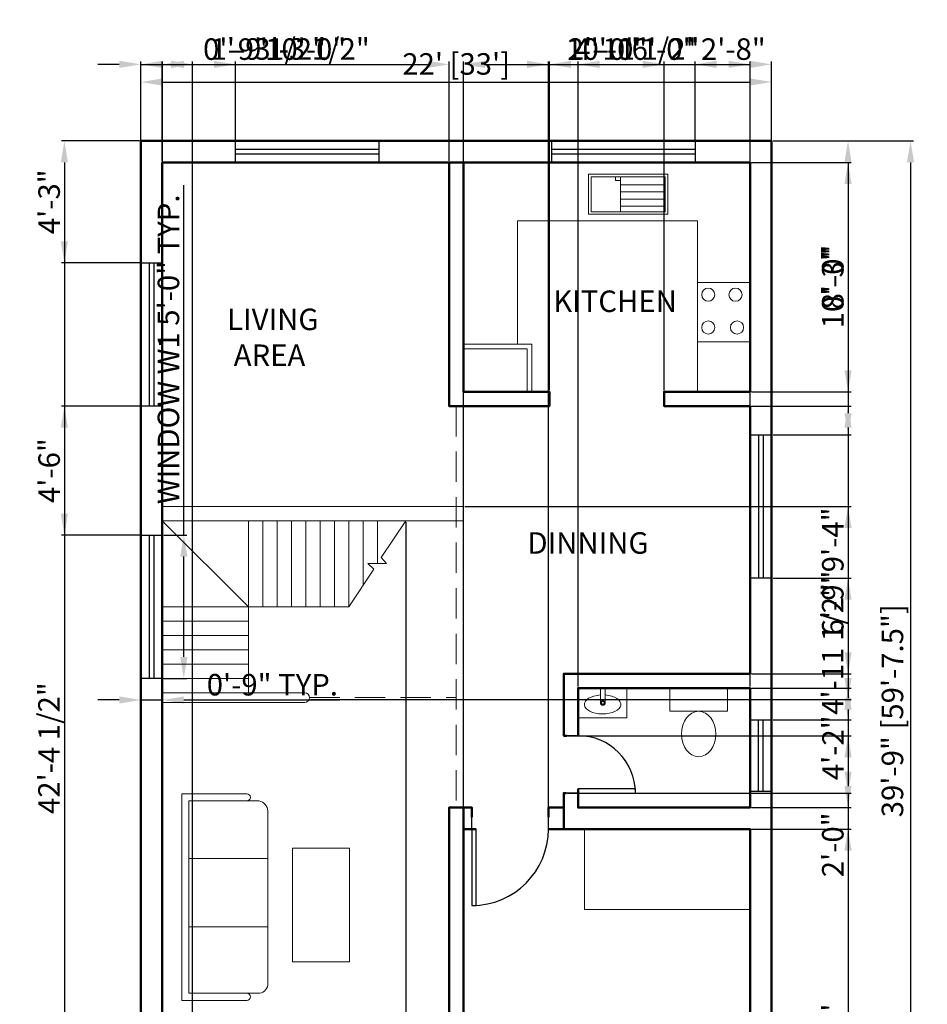
# Model space of a CAD drawing. Units: inches. Extents: x 2429 to 3343, y 1496 to 2530.
# Tile 4 of 7: x 2429 to 2809, y 2118 to 2530. Entities that reach past the tile are written whole.
import ezdxf

# ---------------------------------------------------------------- set-up
doc = ezdxf.new("R2010")
doc.units = ezdxf.units.IN
doc.linetypes.add('DASHED', pattern=[19.05, 12.7, -6.35])
for name, color, linetype, lineweight in [('A-ANNO-DIMS', 2, 'Continuous', 18), ('A-AREA-IDEN', 3, 'Continuous', 18), ('A-DOOR', 3, 'Continuous', 25), ('A-FLOR-FIXT', 8, 'Continuous', 18), ('A-FLOR-OVHD', 8, 'DASHED', 18), ('A-FLOR-STRS', 2, 'Continuous', 18), ('A-FURN', 9, 'Continuous', 18), ('A-GLAZ', 4, 'Continuous', 25), ('A-WALL', 7, 'Continuous', 50)]:
    doc.layers.add(name, color=color, linetype=linetype, lineweight=lineweight)
doc.styles.get("Standard").update_dxf_attribs({"font": 'arial.ttf'})
doc.dimstyles.new('ISO-25', dxfattribs={"dimtxt": 9, "dimasz": 9, "dimexe": 1.25, "dimexo": 0.625, "dimtad": 1, "dimdec": 1, "dimlunit": 3, "dimtxsty": 'Standard', "dimcen": 9, "dimadec": 0, "dimazin": 0, "dimtfac": 1, "dimtdec": 1, "dimtmove": 0, "dimatfit": 3, "dimfxl": 1, "dimarcsym": 0})

# ---------------------------------------------------------------- blocks, each defined once
blk = doc.blocks.new('*U3')
for p, q in [((0, 0), (0, 5)), ((32, 0), (32, 5))]:
    blk.add_line(p, q)
blk.add_lwpolyline([(0, 0), (0, -32), (1.75, -32), (1.75, 0)], close=True)
blk.add_arc((0, 0), 32, 270, 0)
blk = doc.blocks.new('*U4')
for p, q in [((0, 0), (0, 5)), ((24, 0), (24, 5))]:
    blk.add_line(p, q)
blk.add_lwpolyline([(0, 0), (0, -24), (1.75, -24), (1.75, 0)], close=True)
blk.add_arc((0, 0), 24, 270, 0)
blk = doc.blocks.new('*D6')
at = {"layer": 'A-ANNO-DIMS', "color": 0, "lineweight": -2, "transparency": 16777216}
for p, q in [((2479.77, 2480.38), (2479.77, 2505.63)), ((2743.77, 2480.38), (2743.77, 2505.63)), ((2488.77, 2504.38), (2734.77, 2504.38))]:
    blk.add_line(p, q, dxfattribs=at)
at = {"layer": 'A-ANNO-DIMS', "color": 0, "transparency": 16777216}
for points in [[(2488.77, 2505.88), (2488.77, 2502.88), (2479.77, 2504.38)], [(2734.77, 2505.88), (2734.77, 2502.88), (2743.77, 2504.38)]]:
    blk.add_solid(points, dxfattribs=at)
at = {"layer": 'Defpoints', "color": 0, "transparency": 16777216}
for p in [(2743.77, 2504.38), (2479.77, 2479.76), (2743.77, 2479.76)]:
    blk.add_point(p, dxfattribs=at)
at = {"layer": 'A-ANNO-DIMS', "color": 0, "transparency": 16777216, "insert": (2611.77, 2510.77), "char_height": 9, "attachment_point": 5}
blk.add_mtext("22' [33']", dxfattribs=at)
blk = doc.blocks.new('*D7')
at = {"layer": 'A-ANNO-DIMS', "color": 0, "lineweight": -2, "transparency": 16777216}
for p, q in [((2744.82, 2479.76), (2803.17, 2479.76)), ((2801.92, 2470.76), (2801.92, 2011.75)), ((2744.4, 2002.75), (2803.17, 2002.75))]:
    blk.add_line(p, q, dxfattribs=at)
at = {"layer": 'A-ANNO-DIMS', "color": 0, "transparency": 16777216}
for points in [[(2800.42, 2470.76), (2803.42, 2470.76), (2801.92, 2479.76)], [(2800.42, 2011.75), (2803.42, 2011.75), (2801.92, 2002.75)]]:
    blk.add_solid(points, dxfattribs=at)
at = {"layer": 'Defpoints', "color": 0, "transparency": 16777216}
for p in [(2744.19, 2479.76), (2743.77, 2002.75), (2801.92, 2002.75)]:
    blk.add_point(p, dxfattribs=at)
at = {"layer": 'A-ANNO-DIMS', "color": 0, "transparency": 16777216, "insert": (2795.52, 2241.25), "char_height": 9, "attachment_point": 5, "rotation": 90}
blk.add_mtext('39\'-9" [59\'-7.5"]', dxfattribs=at)
blk = doc.blocks.new('WIN-PLAN-1500')
for p, q in [((3.5, 60), (3.5, 0)), ((5.5, 60), (5.5, 0))]:
    blk.add_line(p, q)
blk.add_lwpolyline([(9, 60), (9, 0), (0, 0), (0, 60)], close=True)
blk = doc.blocks.new('WIN-PLAN-750')
for p, q in [((3.5, 0), (3.5, 30)), ((5.5, 0), (5.5, 30))]:
    blk.add_line(p, q)
blk.add_lwpolyline([(9, 30), (9, 0), (0, 0), (0, 30)], close=True)
blk = doc.blocks.new('*D25')
at = {"layer": 'A-ANNO-DIMS', "color": 0, "lineweight": -2, "transparency": 16777216}
for p, q in [((2497.77, 2314.75), (2497.77, 2461.24)), ((2489.4, 2314.75), (2499.02, 2314.75)), ((2497.77, 2263.75), (2497.77, 2305.75)), ((2489.4, 2254.75), (2499.02, 2254.75))]:
    blk.add_line(p, q, dxfattribs=at)
at = {"layer": 'A-ANNO-DIMS', "color": 0, "transparency": 16777216}
for points in [[(2496.27, 2305.75), (2499.27, 2305.75), (2497.77, 2314.75)], [(2496.27, 2263.75), (2499.27, 2263.75), (2497.77, 2254.75)]]:
    blk.add_solid(points, dxfattribs=at)
at = {"layer": 'Defpoints', "color": 0, "transparency": 16777216}
for p in [(2488.77, 2314.75), (2497.77, 2314.75), (2488.77, 2254.75)]:
    blk.add_point(p, dxfattribs=at)
at = {"layer": 'A-ANNO-DIMS', "color": 0, "transparency": 16777216, "insert": (2492.49, 2392.5), "char_height": 9, "attachment_point": 5, "rotation": 90}
blk.add_mtext('WINDOW W1 5\'-0" TYP.', dxfattribs=at)
blk = doc.blocks.new('*D26')
at = {"layer": 'A-ANNO-DIMS', "color": 0, "lineweight": -2, "transparency": 16777216}
for p, q in [((2479.77, 2254.13), (2479.77, 2244.5)), ((2488.77, 2254.13), (2488.77, 2244.5)), ((2470.77, 2245.75), (2461.77, 2245.75)), ((2479.77, 2245.75), (2488.77, 2245.75)), ((2497.77, 2245.75), (2562.88, 2245.75))]:
    blk.add_line(p, q, dxfattribs=at)
at = {"layer": 'A-ANNO-DIMS', "color": 0, "transparency": 16777216}
for points in [[(2470.77, 2247.25), (2470.77, 2244.25), (2479.77, 2245.75)], [(2497.77, 2247.25), (2497.77, 2244.25), (2488.77, 2245.75)]]:
    blk.add_solid(points, dxfattribs=at)
at = {"layer": 'Defpoints', "color": 0, "transparency": 16777216}
for p in [(2479.77, 2254.75), (2488.77, 2254.75), (2488.77, 2245.75)]:
    blk.add_point(p, dxfattribs=at)
at = {"layer": 'A-ANNO-DIMS', "color": 0, "transparency": 16777216, "insert": (2534.83, 2250.97), "char_height": 9, "attachment_point": 5}
blk.add_mtext('0\'-9" TYP.', dxfattribs=at)
blk = doc.blocks.new('*D29')
at = {"layer": 'A-ANNO-DIMS', "color": 0, "lineweight": -2, "transparency": 16777216}
for p, q in [((2479.15, 2479.76), (2446.52, 2479.76)), ((2447.77, 2470.76), (2447.77, 1980.44)), ((2479.15, 1971.44), (2446.52, 1971.44))]:
    blk.add_line(p, q, dxfattribs=at)
at = {"layer": 'A-ANNO-DIMS', "color": 0, "transparency": 16777216}
for points in [[(2446.27, 2470.76), (2449.27, 2470.76), (2447.77, 2479.76)], [(2446.27, 1980.44), (2449.27, 1980.44), (2447.77, 1971.44)]]:
    blk.add_solid(points, dxfattribs=at)
at = {"layer": 'Defpoints', "color": 0, "transparency": 16777216}
for p in [(2479.77, 2479.76), (2447.77, 1971.44), (2479.77, 1971.44)]:
    blk.add_point(p, dxfattribs=at)
at = {"layer": 'A-ANNO-DIMS', "color": 0, "transparency": 16777216, "insert": (2442.49, 2225.6), "char_height": 9, "attachment_point": 5, "rotation": 90}
blk.add_mtext('42\'-4 1/2"', dxfattribs=at)
blk = doc.blocks.new('*D30')
at = {"layer": 'A-ANNO-DIMS', "color": 0, "lineweight": -2, "transparency": 16777216}
for p, q in [((2488.77, 2471.38), (2488.77, 2513.01)), ((2497.77, 2511.76), (2599.77, 2511.76)), ((2608.77, 2471.38), (2608.77, 2513.01))]:
    blk.add_line(p, q, dxfattribs=at)
at = {"layer": 'A-ANNO-DIMS', "color": 0, "transparency": 16777216}
for points in [[(2497.77, 2513.26), (2497.77, 2510.26), (2488.77, 2511.76)], [(2599.77, 2513.26), (2599.77, 2510.26), (2608.77, 2511.76)]]:
    blk.add_solid(points, dxfattribs=at)
at = {"layer": 'Defpoints', "color": 0, "transparency": 16777216}
for p in [(2608.77, 2511.76), (2488.77, 2470.76), (2608.77, 2470.76)]:
    blk.add_point(p, dxfattribs=at)
at = {"layer": 'A-ANNO-DIMS', "color": 0, "transparency": 16777216, "insert": (2548.77, 2516.98), "char_height": 9, "attachment_point": 5}
blk.add_mtext('10\'-0"', dxfattribs=at)
blk = doc.blocks.new('*D31')
at = {"layer": 'A-ANNO-DIMS', "color": 0, "lineweight": -2, "transparency": 16777216}
for p, q in [((2614.77, 2471.38), (2614.77, 2513.01)), ((2623.77, 2511.76), (2725.77, 2511.76)), ((2734.77, 2471.38), (2734.77, 2513.01))]:
    blk.add_line(p, q, dxfattribs=at)
at = {"layer": 'A-ANNO-DIMS', "color": 0, "transparency": 16777216}
for points in [[(2623.77, 2513.26), (2623.77, 2510.26), (2614.77, 2511.76)], [(2725.77, 2513.26), (2725.77, 2510.26), (2734.77, 2511.76)]]:
    blk.add_solid(points, dxfattribs=at)
at = {"layer": 'Defpoints', "color": 0, "transparency": 16777216}
for p in [(2734.77, 2511.76), (2614.77, 2470.76), (2734.77, 2470.76)]:
    blk.add_point(p, dxfattribs=at)
at = {"layer": 'A-ANNO-DIMS', "color": 0, "transparency": 16777216, "insert": (2674.77, 2516.98), "char_height": 9, "attachment_point": 5}
blk.add_mtext('10\'-0"', dxfattribs=at)
blk = doc.blocks.new('*D32')
at = {"layer": 'A-ANNO-DIMS', "color": 0, "lineweight": -2, "transparency": 16777216}
for p, q in [((2735.4, 2470.76), (2777.02, 2470.76)), ((2775.77, 2461.76), (2775.77, 2383.76)), ((2735.4, 2374.76), (2777.02, 2374.76))]:
    blk.add_line(p, q, dxfattribs=at)
at = {"layer": 'A-ANNO-DIMS', "color": 0, "transparency": 16777216}
for points in [[(2774.27, 2461.76), (2777.27, 2461.76), (2775.77, 2470.76)], [(2774.27, 2383.76), (2777.27, 2383.76), (2775.77, 2374.76)]]:
    blk.add_solid(points, dxfattribs=at)
at = {"layer": 'Defpoints', "color": 0, "transparency": 16777216}
for p in [(2734.77, 2470.76), (2734.77, 2374.76), (2775.77, 2374.76)]:
    blk.add_point(p, dxfattribs=at)
at = {"layer": 'A-ANNO-DIMS', "color": 0, "transparency": 16777216, "insert": (2770.55, 2422.76), "char_height": 9, "attachment_point": 5, "rotation": 90}
blk.add_mtext('8\'-0"', dxfattribs=at)
blk = doc.blocks.new('*D33')
at = {"layer": 'A-ANNO-DIMS', "color": 0, "lineweight": -2, "transparency": 16777216}
for p, q in [((2650.77, 2375.38), (2650.77, 2513.01)), ((2659.77, 2511.76), (2689.77, 2511.76)), ((2698.77, 2375.38), (2698.77, 2513.01))]:
    blk.add_line(p, q, dxfattribs=at)
at = {"layer": 'A-ANNO-DIMS', "color": 0, "transparency": 16777216}
for points in [[(2659.77, 2513.26), (2659.77, 2510.26), (2650.77, 2511.76)], [(2689.77, 2513.26), (2689.77, 2510.26), (2698.77, 2511.76)]]:
    blk.add_solid(points, dxfattribs=at)
at = {"layer": 'Defpoints', "color": 0, "transparency": 16777216}
for p in [(2698.77, 2511.76), (2650.77, 2374.76), (2698.77, 2374.76)]:
    blk.add_point(p, dxfattribs=at)
at = {"layer": 'A-ANNO-DIMS', "color": 0, "transparency": 16777216, "insert": (2674.77, 2516.98), "char_height": 9, "attachment_point": 5}
blk.add_mtext('4\'-0"', dxfattribs=at)
blk = doc.blocks.new('*D34')
at = {"layer": 'A-ANNO-DIMS', "color": 0, "lineweight": -2, "transparency": 16777216}
for p, q in [((2590.68, 2320.13), (2590.68, 1870.45)), ((2488.77, 2248.13), (2488.77, 1870.45)), ((2497.77, 1871.7), (2581.68, 1871.7))]:
    blk.add_line(p, q, dxfattribs=at)
at = {"layer": 'A-ANNO-DIMS', "color": 0, "transparency": 16777216}
for points in [[(2497.77, 1873.2), (2497.77, 1870.2), (2488.77, 1871.7)], [(2581.68, 1873.2), (2581.68, 1870.2), (2590.68, 1871.7)]]:
    blk.add_solid(points, dxfattribs=at)
at = {"layer": 'Defpoints', "color": 0, "transparency": 16777216}
for p in [(2590.68, 2320.75), (2488.77, 2248.75), (2590.68, 1871.7)]:
    blk.add_point(p, dxfattribs=at)
at = {"layer": 'A-ANNO-DIMS', "color": 0, "transparency": 16777216, "insert": (2539.73, 1876.92), "char_height": 9, "attachment_point": 5}
blk.add_mtext('8\'-6"', dxfattribs=at)
blk = doc.blocks.new('*D35')
at = {"layer": 'A-ANNO-DIMS', "color": 0, "lineweight": -2, "transparency": 16777216}
for p, q in [((2615.4, 2326.75), (2777.02, 2326.75)), ((2775.77, 2317.75), (2775.77, 2254.97)), ((2550.83, 2245.97), (2777.02, 2245.97))]:
    blk.add_line(p, q, dxfattribs=at)
at = {"layer": 'A-ANNO-DIMS', "color": 0, "transparency": 16777216}
for points in [[(2774.27, 2317.75), (2777.27, 2317.75), (2775.77, 2326.75)], [(2774.27, 2254.97), (2777.27, 2254.97), (2775.77, 2245.97)]]:
    blk.add_solid(points, dxfattribs=at)
at = {"layer": 'Defpoints', "color": 0, "transparency": 16777216}
for p in [(2614.77, 2326.75), (2550.2, 2245.97), (2775.77, 2245.97)]:
    blk.add_point(p, dxfattribs=at)
at = {"layer": 'A-ANNO-DIMS', "color": 0, "transparency": 16777216, "insert": (2770.55, 2286.36), "char_height": 9, "attachment_point": 5, "rotation": 90}
blk.add_mtext('6\'-9"', dxfattribs=at)
blk = doc.blocks.new('*D36')
at = {"layer": 'A-ANNO-DIMS', "color": 0, "lineweight": -2, "transparency": 16777216}
for p, q in [((2662.77, 2251.38), (2662.77, 2513.01)), ((2671.77, 2511.76), (2725.77, 2511.76)), ((2734.77, 2251.38), (2734.77, 2513.01))]:
    blk.add_line(p, q, dxfattribs=at)
at = {"layer": 'A-ANNO-DIMS', "color": 0, "transparency": 16777216}
for points in [[(2671.77, 2513.26), (2671.77, 2510.26), (2662.77, 2511.76)], [(2725.77, 2513.26), (2725.77, 2510.26), (2734.77, 2511.76)]]:
    blk.add_solid(points, dxfattribs=at)
at = {"layer": 'Defpoints', "color": 0, "transparency": 16777216}
for p in [(2734.77, 2511.76), (2662.77, 2250.76), (2734.77, 2250.76)]:
    blk.add_point(p, dxfattribs=at)
at = {"layer": 'A-ANNO-DIMS', "color": 0, "transparency": 16777216, "insert": (2698.77, 2516.98), "char_height": 9, "attachment_point": 5}
blk.add_mtext('6\'-0"', dxfattribs=at)
blk = doc.blocks.new('*D37')
at = {"layer": 'A-ANNO-DIMS', "color": 0, "lineweight": -2, "transparency": 16777216}
for p, q in [((2735.4, 2250.76), (2777.02, 2250.76)), ((2775.77, 2241.76), (2775.77, 2209.75)), ((2735.4, 2200.75), (2777.02, 2200.75))]:
    blk.add_line(p, q, dxfattribs=at)
at = {"layer": 'A-ANNO-DIMS', "color": 0, "transparency": 16777216}
for points in [[(2774.27, 2241.76), (2777.27, 2241.76), (2775.77, 2250.76)], [(2774.27, 2209.75), (2777.27, 2209.75), (2775.77, 2200.75)]]:
    blk.add_solid(points, dxfattribs=at)
at = {"layer": 'Defpoints', "color": 0, "transparency": 16777216}
for p in [(2734.77, 2250.76), (2734.77, 2200.75), (2775.77, 2200.75)]:
    blk.add_point(p, dxfattribs=at)
at = {"layer": 'A-ANNO-DIMS', "color": 0, "transparency": 16777216, "insert": (2770.63, 2225.75), "char_height": 9, "attachment_point": 5, "rotation": 90}
blk.add_mtext('4\'-2"', dxfattribs=at)
blk = doc.blocks.new('*D39')
at = {"layer": 'A-ANNO-DIMS', "color": 0, "lineweight": -2, "transparency": 16777216}
for p, q in [((2735.4, 2191.75), (2777.02, 2191.75)), ((2775.77, 2182.75), (2775.77, 2020.75)), ((2735.4, 2011.75), (2777.02, 2011.75))]:
    blk.add_line(p, q, dxfattribs=at)
at = {"layer": 'A-ANNO-DIMS', "color": 0, "transparency": 16777216}
for points in [[(2774.27, 2182.75), (2777.27, 2182.75), (2775.77, 2191.75)], [(2774.27, 2020.75), (2777.27, 2020.75), (2775.77, 2011.75)]]:
    blk.add_solid(points, dxfattribs=at)
at = {"layer": 'Defpoints', "color": 0, "transparency": 16777216}
for p in [(2734.77, 2191.75), (2734.77, 2011.75), (2775.77, 2011.75)]:
    blk.add_point(p, dxfattribs=at)
at = {"layer": 'A-ANNO-DIMS', "color": 0, "transparency": 16777216, "insert": (2770.55, 2101.75), "char_height": 9, "attachment_point": 5, "rotation": 90}
blk.add_mtext('15\'-0"', dxfattribs=at)
blk = doc.blocks.new('*D40')
at = {"layer": 'A-ANNO-DIMS', "color": 0, "lineweight": -2, "transparency": 16777216}
for p, q in [((2735.4, 2368.76), (2777.02, 2368.76)), ((2775.77, 2359.76), (2775.77, 2265.76)), ((2735.4, 2256.76), (2777.02, 2256.76))]:
    blk.add_line(p, q, dxfattribs=at)
at = {"layer": 'A-ANNO-DIMS', "color": 0, "transparency": 16777216}
for points in [[(2774.27, 2359.76), (2777.27, 2359.76), (2775.77, 2368.76)], [(2774.27, 2265.76), (2777.27, 2265.76), (2775.77, 2256.76)]]:
    blk.add_solid(points, dxfattribs=at)
at = {"layer": 'Defpoints', "color": 0, "transparency": 16777216}
for p in [(2734.77, 2368.76), (2734.77, 2256.76), (2775.77, 2256.76)]:
    blk.add_point(p, dxfattribs=at)
at = {"layer": 'A-ANNO-DIMS', "color": 0, "transparency": 16777216, "insert": (2770.55, 2312.76), "char_height": 9, "attachment_point": 5, "rotation": 90}
blk.add_mtext('9\'-4"', dxfattribs=at)
blk = doc.blocks.new('*D43')
at = {"layer": 'A-ANNO-DIMS', "color": 0, "lineweight": -2, "transparency": 16777216}
for p, q in [((2470.77, 2511.76), (2461.77, 2511.76)), ((2479.77, 1972.06), (2479.77, 2513.01)), ((2479.77, 2511.76), (2488.8, 2511.76)), ((2488.8, 1972.06), (2488.8, 2513.01)), ((2497.8, 2511.76), (2531.97, 2511.76))]:
    blk.add_line(p, q, dxfattribs=at)
at = {"layer": 'A-ANNO-DIMS', "color": 0, "transparency": 16777216}
for points in [[(2470.77, 2513.26), (2470.77, 2510.26), (2479.77, 2511.76)], [(2497.8, 2513.26), (2497.8, 2510.26), (2488.8, 2511.76)]]:
    blk.add_solid(points, dxfattribs=at)
at = {"layer": 'Defpoints', "color": 0, "transparency": 16777216}
for p in [(2488.8, 2511.76), (2479.77, 1971.44), (2488.8, 1971.44)]:
    blk.add_point(p, dxfattribs=at)
at = {"layer": 'A-ANNO-DIMS', "color": 0, "transparency": 16777216, "insert": (2519.38, 2516.98), "char_height": 9, "attachment_point": 5}
blk.add_mtext('0\'-9"', dxfattribs=at)
blk = doc.blocks.new('*D46')
at = {"layer": 'A-ANNO-DIMS', "color": 0, "lineweight": -2, "transparency": 16777216}
for p, q in [((2658.4, 2230.8), (2777.02, 2230.8)), ((2775.77, 2221.8), (2775.77, 2215.8)), ((2658.4, 2206.8), (2777.02, 2206.8)), ((2775.77, 2206.8), (2775.77, 2172.47))]:
    blk.add_line(p, q, dxfattribs=at)
at = {"layer": 'A-ANNO-DIMS', "color": 0, "transparency": 16777216}
for points in [[(2774.27, 2221.8), (2777.27, 2221.8), (2775.77, 2230.8)], [(2774.27, 2215.8), (2777.27, 2215.8), (2775.77, 2206.8)]]:
    blk.add_solid(points, dxfattribs=at)
at = {"layer": 'Defpoints', "color": 0, "transparency": 16777216}
for p in [(2657.77, 2230.8), (2657.77, 2206.8), (2775.77, 2206.8)]:
    blk.add_point(p, dxfattribs=at)
at = {"layer": 'A-ANNO-DIMS', "color": 0, "transparency": 16777216, "insert": (2770.55, 2185.14), "char_height": 9, "attachment_point": 5, "rotation": 90}
blk.add_mtext('2\'-0"', dxfattribs=at)
blk = doc.blocks.new('*D47')
at = {"layer": 'A-ANNO-DIMS', "color": 0, "lineweight": -2, "transparency": 16777216}
for p, q in [((2614.77, 2192.38), (2614.77, 2513.01)), ((2623.77, 2511.76), (2641.37, 2511.76)), ((2650.37, 2192.38), (2650.37, 2513.01)), ((2650.37, 2511.76), (2712.66, 2511.76))]:
    blk.add_line(p, q, dxfattribs=at)
at = {"layer": 'A-ANNO-DIMS', "color": 0, "transparency": 16777216}
for points in [[(2623.77, 2513.26), (2623.77, 2510.26), (2614.77, 2511.76)], [(2641.37, 2513.26), (2641.37, 2510.26), (2650.37, 2511.76)]]:
    blk.add_solid(points, dxfattribs=at)
at = {"layer": 'Defpoints', "color": 0, "transparency": 16777216}
for p in [(2650.37, 2511.76), (2614.77, 2191.75), (2650.37, 2191.75)]:
    blk.add_point(p, dxfattribs=at)
at = {"layer": 'A-ANNO-DIMS', "color": 0, "transparency": 16777216, "insert": (2686.01, 2517.03), "char_height": 9, "attachment_point": 5}
blk.add_mtext('2\'-11 1/2"', dxfattribs=at)
blk = doc.blocks.new('*D48')
at = {"layer": 'A-ANNO-DIMS', "color": 0, "lineweight": -2, "transparency": 16777216}
for p, q in [((2479.77, 2480.38), (2479.77, 2513.01)), ((2488.77, 2511.76), (2510.36, 2511.76)), ((2519.36, 2480.38), (2519.36, 2513.01)), ((2519.36, 2511.76), (2574.5, 2511.76))]:
    blk.add_line(p, q, dxfattribs=at)
at = {"layer": 'A-ANNO-DIMS', "color": 0, "transparency": 16777216}
for points in [[(2488.77, 2513.26), (2488.77, 2510.26), (2479.77, 2511.76)], [(2510.36, 2513.26), (2510.36, 2510.26), (2519.36, 2511.76)]]:
    blk.add_solid(points, dxfattribs=at)
at = {"layer": 'Defpoints', "color": 0, "transparency": 16777216}
for p in [(2519.36, 2511.76), (2479.77, 2479.76), (2519.36, 2479.76)]:
    blk.add_point(p, dxfattribs=at)
at = {"layer": 'A-ANNO-DIMS', "color": 0, "transparency": 16777216, "insert": (2551.43, 2517.04), "char_height": 9, "attachment_point": 5}
blk.add_mtext('3\'-3 1/2"', dxfattribs=at)
blk = doc.blocks.new('*D49')
at = {"layer": 'A-ANNO-DIMS', "color": 0, "lineweight": -2, "transparency": 16777216}
for p, q in [((2711.73, 2480.38), (2711.73, 2513.01)), ((2720.73, 2511.76), (2734.77, 2511.76)), ((2743.77, 2480.38), (2743.77, 2513.01))]:
    blk.add_line(p, q, dxfattribs=at)
at = {"layer": 'A-ANNO-DIMS', "color": 0, "transparency": 16777216}
for points in [[(2720.73, 2513.26), (2720.73, 2510.26), (2711.73, 2511.76)], [(2734.77, 2513.26), (2734.77, 2510.26), (2743.77, 2511.76)]]:
    blk.add_solid(points, dxfattribs=at)
at = {"layer": 'Defpoints', "color": 0, "transparency": 16777216}
for p in [(2743.77, 2511.76), (2711.73, 2479.76), (2743.77, 2479.76)]:
    blk.add_point(p, dxfattribs=at)
at = {"layer": 'A-ANNO-DIMS', "color": 0, "transparency": 16777216, "insert": (2727.75, 2516.98), "char_height": 9, "attachment_point": 5}
blk.add_mtext('2\'-8"', dxfattribs=at)
blk = doc.blocks.new('*D50')
at = {"layer": 'A-ANNO-DIMS', "color": 0, "lineweight": -2, "transparency": 16777216}
for p, q in [((2479.15, 2479.76), (2446.52, 2479.76)), ((2447.77, 2470.76), (2447.77, 2437.75)), ((2479.15, 2428.75), (2446.52, 2428.75))]:
    blk.add_line(p, q, dxfattribs=at)
at = {"layer": 'A-ANNO-DIMS', "color": 0, "transparency": 16777216}
for points in [[(2446.27, 2470.76), (2449.27, 2470.76), (2447.77, 2479.76)], [(2446.27, 2437.75), (2449.27, 2437.75), (2447.77, 2428.75)]]:
    blk.add_solid(points, dxfattribs=at)
at = {"layer": 'Defpoints', "color": 0, "transparency": 16777216}
for p in [(2479.77, 2479.76), (2447.77, 2428.75), (2479.77, 2428.75)]:
    blk.add_point(p, dxfattribs=at)
at = {"layer": 'A-ANNO-DIMS', "color": 0, "transparency": 16777216, "insert": (2442.55, 2454.25), "char_height": 9, "attachment_point": 5, "rotation": 90}
blk.add_mtext('4\'-3"', dxfattribs=at)
blk = doc.blocks.new('*D51')
at = {"layer": 'A-ANNO-DIMS', "color": 0, "lineweight": -2, "transparency": 16777216}
for p, q in [((2479.15, 2368.75), (2446.52, 2368.75)), ((2447.77, 2359.75), (2447.77, 2323.75)), ((2479.15, 2314.75), (2446.52, 2314.75))]:
    blk.add_line(p, q, dxfattribs=at)
at = {"layer": 'A-ANNO-DIMS', "color": 0, "transparency": 16777216}
for points in [[(2446.27, 2359.75), (2449.27, 2359.75), (2447.77, 2368.75)], [(2446.27, 2323.75), (2449.27, 2323.75), (2447.77, 2314.75)]]:
    blk.add_solid(points, dxfattribs=at)
at = {"layer": 'Defpoints', "color": 0, "transparency": 16777216}
for p in [(2479.77, 2368.75), (2447.77, 2314.75), (2479.77, 2314.75)]:
    blk.add_point(p, dxfattribs=at)
at = {"layer": 'A-ANNO-DIMS', "color": 0, "transparency": 16777216, "insert": (2442.55, 2341.75), "char_height": 9, "attachment_point": 5, "rotation": 90}
blk.add_mtext('4\'-6"', dxfattribs=at)
blk = doc.blocks.new('*D52')
at = {"layer": 'A-ANNO-DIMS', "color": 0, "lineweight": -2, "transparency": 16777216}
for p, q in [((2744.4, 2479.76), (2777.02, 2479.76)), ((2775.77, 2470.76), (2775.77, 2365.75)), ((2744.4, 2356.75), (2777.02, 2356.75))]:
    blk.add_line(p, q, dxfattribs=at)
at = {"layer": 'A-ANNO-DIMS', "color": 0, "transparency": 16777216}
for points in [[(2774.27, 2470.76), (2777.27, 2470.76), (2775.77, 2479.76)], [(2774.27, 2365.75), (2777.27, 2365.75), (2775.77, 2356.75)]]:
    blk.add_solid(points, dxfattribs=at)
at = {"layer": 'Defpoints', "color": 0, "transparency": 16777216}
for p in [(2743.77, 2479.76), (2743.77, 2356.75), (2775.77, 2356.75)]:
    blk.add_point(p, dxfattribs=at)
at = {"layer": 'A-ANNO-DIMS', "color": 0, "transparency": 16777216, "insert": (2770.55, 2418.25), "char_height": 9, "attachment_point": 5, "rotation": 90}
blk.add_mtext('10\'-3"', dxfattribs=at)
blk = doc.blocks.new('*D53')
at = {"layer": 'A-ANNO-DIMS', "color": 0, "lineweight": -2, "transparency": 16777216}
for p, q in [((2744.4, 2296.75), (2777.02, 2296.75)), ((2775.77, 2287.75), (2775.77, 2246.46)), ((2744.4, 2237.46), (2777.02, 2237.46))]:
    blk.add_line(p, q, dxfattribs=at)
at = {"layer": 'A-ANNO-DIMS', "color": 0, "transparency": 16777216}
for points in [[(2774.27, 2287.75), (2777.27, 2287.75), (2775.77, 2296.75)], [(2774.27, 2246.46), (2777.27, 2246.46), (2775.77, 2237.46)]]:
    blk.add_solid(points, dxfattribs=at)
at = {"layer": 'Defpoints', "color": 0, "transparency": 16777216}
for p in [(2743.77, 2296.75), (2743.77, 2237.46), (2775.77, 2237.46)]:
    blk.add_point(p, dxfattribs=at)
at = {"layer": 'A-ANNO-DIMS', "color": 0, "transparency": 16777216, "insert": (2770.49, 2267.11), "char_height": 9, "attachment_point": 5, "rotation": 90}
blk.add_mtext('4\'-11 1/2"', dxfattribs=at)
blk = doc.blocks.new('*D54')
at = {"layer": 'A-ANNO-DIMS', "color": 0, "lineweight": -2, "transparency": 16777216}
for p, q in [((2479.77, 2072.38), (2479.77, 2513.01)), ((2488.77, 2511.76), (2492.46, 2511.76)), ((2501.46, 2072.38), (2501.46, 2513.01)), ((2501.46, 2511.76), (2555.76, 2511.76))]:
    blk.add_line(p, q, dxfattribs=at)
at = {"layer": 'A-ANNO-DIMS', "color": 0, "transparency": 16777216}
for points in [[(2488.77, 2513.26), (2488.77, 2510.26), (2479.77, 2511.76)], [(2492.46, 2513.26), (2492.46, 2510.26), (2501.46, 2511.76)]]:
    blk.add_solid(points, dxfattribs=at)
at = {"layer": 'Defpoints', "color": 0, "transparency": 16777216}
for p in [(2501.46, 2511.76), (2479.77, 2071.75), (2501.46, 2071.75)]:
    blk.add_point(p, dxfattribs=at)
at = {"layer": 'A-ANNO-DIMS', "color": 0, "transparency": 16777216, "insert": (2533.11, 2517.03), "char_height": 9, "attachment_point": 5}
blk.add_mtext('1\'-9 1/2"', dxfattribs=at)

msp = doc.modelspace()

# ---------------------------------------------------------------- hatches: boundary and pattern name
at = {"layer": 'A-FLOR-FIXT'}
h = msp.add_hatch(color=256, dxfattribs=at)
h.dxf.hatch_style = 1
h.paths.add_polyline_path([(2672.14515, 2244.52848, 1), (2674.14515, 2244.52848, 1)])
h.paths.add_polyline_path([(2673.70762, 2244.52848, -1), (2672.58269, 2244.52848, -1)], flags=16)

# ---------------------------------------------------------------- linework, layer by layer
for p, q in [((2680.59018, 2464.75512), (2680.59018, 2450.02691)), ((2680.59018, 2461.38243), (2699.28813, 2461.38243)), ((2680.59018, 2458.38243), (2699.28813, 2458.38243)), ((2680.59018, 2455.38243), (2699.28813, 2455.38243)), ((2680.59018, 2452.38243), (2699.28813, 2452.38243)), ((2712.77109, 2420.52216), (2734.77257, 2420.52216)), ((2712.77109, 2395.6064), (2734.77257, 2395.6064))]:
    msp.add_line(p, q, dxfattribs=at)
for points in [[(2667.19363, 2465.75512), (2700.28813, 2465.75512), (2700.28813, 2449.02691), (2667.19363, 2449.02691)], [(2668.19363, 2464.75512), (2699.28813, 2464.75512), (2699.28813, 2450.02691), (2668.19363, 2450.02691)]]:
    msp.add_lwpolyline(points, close=True, dxfattribs=at)
for points in [[(2678.4916, 2464.75512), (2678.4916, 2463.12164), (2680.59018, 2463.12164)], [(2637.41644, 2394.64579), (2637.41644, 2446.29538), (2712.77109, 2446.29538), (2712.77109, 2374.75602)], [(2662.77257, 2238.21467), (2683.19871, 2238.21467), (2683.19871, 2250.75602)], [(2701.18915, 2250.75602), (2701.18915, 2241.03426), (2725.29415, 2241.03426), (2725.29415, 2250.75602)]]:
    msp.add_lwpolyline(points, dxfattribs=at)
msp.add_lwpolyline([(2672.14515, 2250.75602), (2672.14515, 2244.52848, 1), (2674.14515, 2244.52848), (2674.14515, 2250.75602)], format="xyb", dxfattribs=at)
for centre, radius in [((2717.26639, 2415.37019), 2.74723), ((2728.64581, 2415.37019), 2.74723), ((2717.26639, 2401.63403), 2.74723), ((2729.30948, 2401.63403), 2.74723), ((2673.14515, 2244.52848), 1), ((2673.14515, 2244.52848), 0.56247)]:
    msp.add_circle(centre, radius, dxfattribs=at)
msp.add_ellipse((2673.03582, 2243.89542), major_axis=(7.63165, 0), ratio=0.522688861, start_param=1.687769865, end_param=7.708105138, dxfattribs=at)
msp.add_ellipse((2713.24165, 2231.5072), major_axis=(0, -9.52707), ratio=0.757824975, dxfattribs=at)
at = {"layer": 'A-FLOR-OVHD'}
for p, q in [((2611.77257, 2368.75602), (2611.77257, 2200.7507)), ((2550.35753, 2246.7507), (2611.77257, 2246.7507))]:
    msp.add_line(p, q, dxfattribs=at)
at = {"layer": 'A-FLOR-STRS'}
for p, q in [((2524.77257, 2248.7507), (2524.77257, 2320.7507)), ((2530.77257, 2284.7507), (2530.77257, 2320.7507)), ((2536.77257, 2284.7507), (2536.77257, 2320.7507)), ((2542.77257, 2284.7507), (2542.77257, 2320.7507)), ((2548.77257, 2284.7507), (2548.77257, 2320.7507)), ((2554.77257, 2284.7507), (2554.77257, 2320.7507)), ((2560.77257, 2284.7507), (2560.77257, 2320.7507)), ((2572.77257, 2293.78539), (2572.77257, 2320.7507)), ((2566.77257, 2284.7507), (2488.77257, 2284.7507)), ((2488.77257, 2278.7507), (2524.77257, 2278.7507)), ((2488.77257, 2272.7507), (2524.77257, 2272.7507)), ((2488.77257, 2266.7507), (2524.77257, 2266.7507)), ((2488.77257, 2260.7507), (2524.77257, 2260.7507)), ((2488.77257, 2254.7507), (2524.77257, 2254.7507))]:
    msp.add_line(p, q, dxfattribs=at)
for points in [[(2488.77257, 2326.7507), (2608.77257, 2326.7507), (2614.77257, 2326.7507), (2614.77257, 2320.7507), (2488.77257, 2320.7507), (2524.77257, 2284.7507)], [(2578.77257, 2302.82009), (2574.83944, 2302.82009), (2577.24521, 2300.52021), (2566.77257, 2284.7507), (2566.77257, 2320.7507)], [(2578.77257, 2320.7507), (2578.77257, 2302.82009), (2582.63541, 2302.82009), (2580.43357, 2305.32118), (2590.68041, 2320.7507)]]:
    msp.add_lwpolyline(points, dxfattribs=at)
msp.add_lwpolyline([(2488.77257, 2244.7507), (2548.35753, 2244.7507, 1), (2548.35753, 2248.7507), (2488.77257, 2248.7507)], format="xyb", dxfattribs=at)
at = {"layer": 'A-FURN'}
for p, q in [((2499.92065, 2179.38597), (2532.90986, 2179.38597)), ((2499.92065, 2150.7572), (2532.90986, 2150.7572))]:
    msp.add_line(p, q, dxfattribs=at)
for points in [[(2614.77257, 2394.64579), (2643.4489, 2394.64579), (2643.4489, 2374.75602)], [(2614.77257, 2392.64579), (2641.4489, 2392.64579), (2641.4489, 2374.75602)], [(2665.49179, 2191.7507), (2665.49179, 2158.06801), (2734.77257, 2158.06801)]]:
    msp.add_lwpolyline(points, dxfattribs=at)
for points in [[(2524.1217, 2123.03037), (2499.92065, 2123.03037), (2499.92065, 2203.50803), (2524.1217, 2203.50803, 1), (2524.1217, 2206.50803), (2496.92065, 2206.50803), (2496.92065, 2120.03037), (2524.1217, 2120.03037, 1), (2524.1217, 2123.03037), (2529.24812, 2123.03037)], [(2528.76628, 2123.03037, 0.3909175), (2532.90986, 2126.40966), (2532.90986, 2199.29265, 0.341849533), (2529.27871, 2203.50803), (2520.63409, 2203.50803)]]:
    msp.add_lwpolyline(points, format="xyb", dxfattribs=at)
msp.add_lwpolyline([(2543.28451, 2183.72972), (2567.11852, 2183.72972), (2567.11852, 2136.10076), (2543.28451, 2136.10076)], close=True, dxfattribs=at)
at = {"layer": 'A-WALL'}
for points in [[(2603.44497, 2075.7507), (2603.44497, 2071.7507), (2608.77257, 2071.7507), (2608.77257, 2002.7507), (2743.77257, 2002.7507), (2743.77257, 2326.7507), (2743.77257, 2479.75602), (2479.77257, 2479.75602), (2479.77257, 2326.7507), (2479.77257, 2320.7507), (2479.77257, 2200.7507), (2479.77257, 2071.7507), (2567.44497, 2071.7507), (2567.44497, 2073.04361), (2567.44497, 2075.7507)], [(2658.07657, 2230.80141), (2656.77257, 2230.80141), (2656.77257, 2256.75602), (2734.77257, 2256.75602), (2734.77257, 2326.7507), (2734.77257, 2368.75602), (2698.77257, 2368.75602), (2698.77257, 2374.75602), (2734.77257, 2374.75602), (2734.77257, 2470.75602), (2488.77257, 2470.75602), (2488.77257, 2326.7507), (2488.77257, 2320.7507), (2488.77257, 2200.7507), (2488.77257, 2080.7507), (2567.44497, 2080.7507)], [(2614.77257, 2470.75602), (2614.77257, 2374.75602), (2650.77257, 2374.75602), (2650.77257, 2368.75602), (2614.77257, 2368.75602), (2608.77257, 2368.75602), (2608.77257, 2470.75602)], [(2662.77257, 2230.80141), (2662.77257, 2250.75602), (2734.77257, 2250.75602), (2734.77257, 2200.7507), (2662.77257, 2200.7507), (2662.77257, 2208.55141)], [(2656.77257, 2191.7507), (2656.77257, 2206.80141), (2657.77257, 2206.80141)], [(2601.69497, 2080.7507), (2608.77257, 2080.7507), (2608.77257, 2200.7507), (2614.77257, 2200.7507)], [(2620.11679, 2191.7507), (2614.77257, 2191.7507), (2614.77257, 2200.7507), (2618.36679, 2200.7507), (2618.36679, 2196.7507)], [(2650.36679, 2196.7507), (2650.36679, 2200.7507), (2656.77257, 2200.7507)], [(2614.77257, 2191.7507), (2614.77257, 2071.7507), (2617.77257, 2071.7507), (2617.77257, 2011.7507), (2734.77257, 2011.7507), (2734.77257, 2191.7507), (2650.36679, 2191.7507)]]:
    msp.add_lwpolyline(points, dxfattribs=at)

# ---------------------------------------------------------------- block references
at = {"layer": 'A-DOOR', "rotation": 90}
msp.add_blockref('*U4', (2662.77257, 2206.80141), dxfattribs=at)
at = {"layer": 'A-DOOR'}
msp.add_blockref('*U3', (2618.36679, 2191.7507), dxfattribs=at)
at = {"layer": 'A-GLAZ', "rotation": 90.00000000000011}
for p in [(2579.36386, 2470.75645), (2711.73359, 2470.75645)]:
    msp.add_blockref('WIN-PLAN-1500', p, dxfattribs=at)
at = {"layer": 'A-GLAZ'}
for name, p in [('WIN-PLAN-1500', (2479.773, 2368.753)), ('WIN-PLAN-1500', (2734.773, 2296.75034)), ('WIN-PLAN-1500', (2479.773, 2254.75034)), ('WIN-PLAN-750', (2734.773, 2207.464))]:
    msp.add_blockref(name, p, dxfattribs=at)

# ---------------------------------------------------------------- texts
at = {"layer": 'A-AREA-IDEN', "char_height": 9, "attachment_point": 1}
for s, width, insert in [('{\\fCalibri|b0|i0|c0|p34;KITCHEN}', 51.2251285, (2652.36906, 2417.12566)), ('{\\fCalibri|b0|i0|c0|p34; LIVING \\P  AREA}', 73.2771466, (2513.15122, 2409.53104)), ('{\\fCalibri|b0|i0|c0|p34;DINNING}', 73.2771466, (2641.58567, 2315.9576))]:
    msp.add_mtext_dynamic_manual_height_columns(s, width=width, gutter_width=12.5, heights=[0], dxfattribs=dict(at, insert=insert))

# ---------------------------------------------------------------- dimensions: what is measured, and where the dimension line sits
at = {"layer": 'A-ANNO-DIMS'}
for base, p1, p2, override, picture, middle in [((2519.3635, 2511.75602), (2479.77257, 2479.75602), (2519.3635, 2479.75602), {"dimdec": 1, "dimlfac": 1, "dimrnd": 0, "dimzin": 1, "dimdsep": 46, "dimlunit": 4, "dimfrac": 2}, '*D48', (2551.43324, 2517.03757)), ((2501.45753, 2511.75602), (2479.77257, 2071.7507), (2501.45753, 2071.7507), {"dimdec": 1, "dimlfac": 1, "dimrnd": 0, "dimzin": 1, "dimdsep": 46, "dimlunit": 4, "dimfrac": 2}, '*D54', (2533.10674, 2517.0345)), ((2650.36679, 2511.75602), (2614.77257, 2191.7507), (2650.36679, 2191.7507), {"dimdec": 1, "dimlfac": 1, "dimrnd": 0, "dimzin": 1, "dimdsep": 46, "dimlunit": 4, "dimfrac": 2}, '*D47', (2686.01259, 2517.0345)), ((2488.79617, 2511.75602), (2479.77257, 1971.43605), (2488.79617, 1971.43605), {"dimdec": 1, "dimlfac": 1, "dimrnd": 0, "dimzin": 1, "dimdsep": 46, "dimlunit": 4, "dimfrac": 2}, '*D43', (2519.38331, 2516.97617)), ((2743.77257, 2504.37968), (2479.77257, 2479.75602), (2743.77257, 2479.75602), {"dimclrd": 0, "dimclre": 0, "dimclrt": 0}, '*D6', (2611.77257, 2510.77241)), ((2608.77257, 2511.75602), (2488.77257, 2470.75602), (2608.77257, 2470.75602), {"dimdec": 1, "dimlfac": 1, "dimrnd": 0, "dimzin": 1, "dimdsep": 46, "dimlunit": 4, "dimfrac": 2}, '*D30', (2548.77257, 2516.97617)), ((2734.77257, 2511.75602), (2614.77257, 2470.75602), (2734.77257, 2470.75602), {"dimdec": 1, "dimlfac": 1, "dimrnd": 0, "dimzin": 1, "dimdsep": 46, "dimlunit": 4, "dimfrac": 2}, '*D31', (2674.77257, 2516.97617)), ((2698.77257, 2511.75602), (2650.77257, 2374.75602), (2698.77257, 2374.75602), {"dimdec": 1, "dimlfac": 1, "dimrnd": 0, "dimzin": 1, "dimdsep": 46, "dimlunit": 4, "dimfrac": 2}, '*D33', (2674.77257, 2516.97617)), ((2734.77257, 2511.75602), (2662.77257, 2250.75602), (2734.77257, 2250.75602), {"dimdec": 1, "dimlfac": 1, "dimrnd": 0, "dimzin": 1, "dimdsep": 46, "dimlunit": 4, "dimfrac": 2}, '*D36', (2698.77257, 2516.97617)), ((2743.77257, 2511.75602), (2711.73323, 2479.75602), (2743.77257, 2479.75602), {"dimdec": 1, "dimlfac": 1, "dimrnd": 0, "dimzin": 1, "dimdsep": 46, "dimlunit": 4, "dimfrac": 2}, '*D49', (2727.7529, 2516.97617)), ((2590.68041, 1871.69967), (2488.77257, 2248.7507), (2590.68041, 2320.7507), {"dimdec": 1, "dimlfac": 1, "dimrnd": 0, "dimzin": 1, "dimdsep": 46, "dimlunit": 4, "dimfrac": 2}, '*D34', (2539.72649, 1876.91983))]:
    dim = msp.add_linear_dim(base=base, p1=p1, p2=p2, dimstyle='ISO-25', override=override, dxfattribs=at)
    dim.commit()
    dim.dimension.update_dxf_attribs({"geometry": picture, "text_midpoint": middle})
for base, p1, p2, override, picture, middle in [((2447.77257, 1971.43605), (2479.77257, 2479.75602), (2479.77257, 1971.43605), {"dimdec": 1, "dimlfac": 1, "dimrnd": 0, "dimzin": 1, "dimdsep": 46, "dimlunit": 4, "dimfrac": 2}, '*D29', (2442.49409, 2225.59604)), ((2447.77257, 2428.75336), (2479.77257, 2479.75602), (2479.77257, 2428.75336), {"dimdec": 1, "dimlfac": 1, "dimrnd": 0, "dimzin": 1, "dimdsep": 46, "dimlunit": 4, "dimfrac": 2}, '*D50', (2442.54935, 2454.25469)), ((2801.91709, 2002.7507), (2744.19025, 2479.75602), (2743.77257, 2002.7507), {"dimclrd": 0, "dimclre": 0, "dimclrt": 0}, '*D7', (2795.52436, 2241.25336)), ((2775.77257, 2356.7507), (2743.77257, 2479.75602), (2743.77257, 2356.7507), {"dimdec": 1, "dimlfac": 1, "dimrnd": 0, "dimzin": 1, "dimdsep": 46, "dimlunit": 4, "dimfrac": 2}, '*D52', (2770.54935, 2418.25336)), ((2775.77257, 2374.75602), (2734.77257, 2470.75602), (2734.77257, 2374.75602), {"dimdec": 1, "dimlfac": 1, "dimrnd": 0, "dimzin": 1, "dimdsep": 46, "dimlunit": 4, "dimfrac": 2}, '*D32', (2770.55242, 2422.75602)), ((2447.77257, 2314.7507), (2479.77257, 2368.75336), (2479.77257, 2314.7507), {"dimdec": 1, "dimlfac": 1, "dimrnd": 0, "dimzin": 1, "dimdsep": 46, "dimlunit": 4, "dimfrac": 2}, '*D51', (2442.55242, 2341.75203)), ((2775.77257, 2256.75602), (2734.77257, 2368.75602), (2734.77257, 2256.75602), {"dimdec": 1, "dimlfac": 1, "dimrnd": 0, "dimzin": 1, "dimdsep": 46, "dimlunit": 4, "dimfrac": 2}, '*D40', (2770.55242, 2312.75602)), ((2775.77257, 2245.97221), (2614.77257, 2326.7507), (2550.20036, 2245.97221), {"dimdec": 1, "dimlfac": 1, "dimrnd": 0, "dimzin": 1, "dimdsep": 46, "dimlunit": 4, "dimfrac": 2}, '*D35', (2770.55242, 2286.36146)), ((2775.77257, 2237.46438), (2743.77257, 2296.7507), (2743.77257, 2237.46438), {"dimdec": 1, "dimlfac": 1, "dimrnd": 0, "dimzin": 1, "dimdsep": 46, "dimlunit": 4, "dimfrac": 2}, '*D53', (2770.49409, 2267.10754)), ((2775.77257, 2200.7507), (2734.77257, 2250.75602), (2734.77257, 2200.7507), {"dimdec": 1, "dimlfac": 1, "dimrnd": 0, "dimzin": 1, "dimdsep": 46, "dimlunit": 4, "dimfrac": 2}, '*D37', (2770.62916, 2225.75336)), ((2775.77257, 2206.80141), (2657.77257, 2230.80141), (2657.77257, 2206.80141), {"dimdec": 1, "dimlfac": 1, "dimrnd": 0, "dimzin": 1, "dimdsep": 46, "dimlunit": 4, "dimfrac": 2}, '*D46', (2770.55242, 2185.13753)), ((2775.77257, 2011.7507), (2734.77257, 2191.7507), (2734.77257, 2011.7507), {"dimdec": 1, "dimlfac": 1, "dimrnd": 0, "dimzin": 1, "dimdsep": 46, "dimlunit": 4, "dimfrac": 2}, '*D39', (2770.55242, 2101.7507))]:
    dim = msp.add_linear_dim(base=base, p1=p1, p2=p2, angle=90, dimstyle='ISO-25', override=override, dxfattribs=at)
    dim.commit()
    dim.dimension.update_dxf_attribs({"geometry": picture, "text_midpoint": middle})
dim = msp.add_linear_dim(base=(2497.77257, 2314.7507), p1=(2488.77257, 2254.7507), p2=(2488.77257, 2314.7507), angle=90, text='WINDOW W1 <> TYP.', dimstyle='ISO-25', override={"dimdec": 1, "dimlfac": 1, "dimrnd": 0, "dimzin": 1, "dimdsep": 46, "dimlunit": 4, "dimfrac": 2}, dxfattribs=at)
dim.commit()
dim.dimension.update_dxf_attribs({"geometry": '*D25', "text_midpoint": (2492.49102, 2392.49576)})
dim = msp.add_linear_dim(base=(2488.77257, 2245.7507), p1=(2479.77257, 2254.7507), p2=(2488.77257, 2254.7507), text='<> TYP.', dimstyle='ISO-25', override={"dimdec": 1, "dimlfac": 1, "dimrnd": 0, "dimzin": 1, "dimdsep": 46, "dimlunit": 4, "dimfrac": 2}, dxfattribs=at)
dim.commit()
dim.dimension.update_dxf_attribs({"geometry": '*D26', "text_midpoint": (2534.82731, 2250.97086)})

doc.saveas('drawing.dxf')
